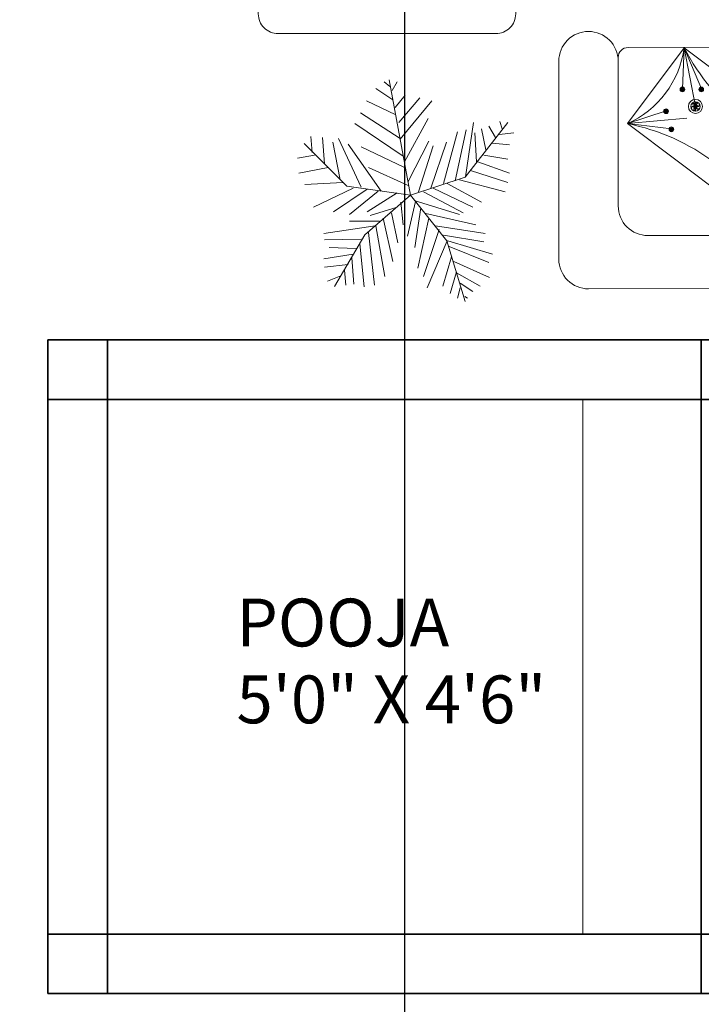
# Model space of a CAD drawing. Units: inches. Extents: x -61 to 1599, y -1316 to 257.
# Tile 22 of 204: x 365 to 434, y -1011 to -912. Entities that reach past the tile are written whole.
import ezdxf

# ---------------------------------------------------------------- set-up
doc = ezdxf.new("R2010")
doc.units = ezdxf.units.IN
doc.header["$MEASUREMENT"] = 0
for name, color, linetype, lineweight in [('A-ANNO-DIMS', 2, 'Continuous', 18), ('A-AREA-IDEN', 1, 'Continuous', 18), ('A-FLOR-CASE', 8, 'Continuous', 18), ('FURNITURE', 83, 'Continuous', 18), ('WALLS', 4, 'Continuous', 35)]:
    doc.layers.add(name, color=color, linetype=linetype, lineweight=lineweight)
doc.layers.add('FUR', color=83, linetype='Continuous')
doc.styles.get("Standard").update_dxf_attribs({"font": 'arial.ttf'})
doc.dimstyles.get("Standard").update_dxf_attribs({"dimtxt": 0.18, "dimasz": 0.18, "dimexe": 0.18, "dimexo": 0.0625, "dimgap": 0.09, "dimtad": 0, "dimtih": 1, "dimtoh": 1, "dimdec": 0, "dimzin": 0, "dimdsep": 46, "dimlunit": 3, "dimtxsty": 'Standard', "dimcen": 0.09, "dimadec": 0, "dimazin": 0, "dimtfac": 1, "dimtdec": 0, "dimtofl": 0, "dimtmove": 0, "dimatfit": 3, "dimfxl": 1, "dimtolj": 1, "dimtzin": 0, "dimarcsym": 0})

# ---------------------------------------------------------------- blocks, each defined once
blk = doc.blocks.new('*U264')
for p, q in [((-10.186, 53.64), (-13.084, 55.962)), ((0, 0), (-10.5, 57)), ((-9.099, 51.782), (-6.563, 55.962)), ((-8.737, 47.138), (-17.069, 52.711)), ((-7.65, 43.423), (-2.578, 49.46)), ((-7.288, 39.707), (-21.778, 46.673)), ((-5.839, 35.992), (4.667, 48.067)), ((-5.114, 27.632), (10.463, 46.673)), ((-5.114, 28.097), (-24.676, 40.636)), ((-3.665, 19.273), (-27.574, 35.527)), ((-2.941, 16.486), (8.652, 37.85)), ((27, 9), (48, 36)), ((27.127, 9.056), (31.112, 35.992)), ((38.719, 34.134), (41.979, 28.561)), ((44.153, 36.456), (45.239, 32.741)), ((16.259, 5.805), (23.142, 31.348)), ((22.055, 7.198), (27.489, 32.277)), ((31.836, 30.883), (32.561, 16.486)), ((35.096, 32.741), (37.27, 22.524)), ((43.791, 29.954), (51.036, 30.883)), ((-31.5, 4.5), (-52.5, 25.5)), ((-48.585, 21.131), (-49.309, 29.026)), ((-43.513, 28.561), (-42.427, 15.558)), ((-38.442, 26.239), (-34.819, 7.663)), ((-35.544, 28.097), (-24.314, 3.947)), ((-14.533, 2.09), (-30.834, 25.31)), ((-1.129, 6.734), (9.014, 26.704)), ((3.942, 1.625), (11.187, 24.381)), ((10.101, 3.483), (17.708, 26.239)), ((40.53, 25.775), (48.862, 24.846)), ((-47.498, 19.737), (-55.83, 18.344)), ((-24.314, 23.917), (-2.941, 13.7)), ((36.183, 19.737), (48.137, 17.88)), ((33.285, 16.486), (48.862, 10.913)), ((-40.615, 13.7), (-55.105, 10.913)), ((-20.691, 13.7), (-1.129, 4.876)), ((29.662, 12.307), (48.137, 6.269)), ((-33.37, 6.269), (-52.207, 5.34)), ((0, 0), (27, 9)), ((18.07, 5.805), (35.096, -3.483)), ((24.229, 7.663), (46.688, 1.625)), ((-28.299, 3.483), (-47.86, -5.805)), ((-21.416, 3.018), (-38.079, -8.128)), ((0, 0), (-31.5, 4.5)), ((-15.982, 2.09), (-30.11, -9.521)), ((0, 0), (-22.5, -19.5)), ((-6.563, 1.161), (-21.416, -8.128)), ((0, 0), (18, -22.5)), ((6.478, 1.625), (26.04, -8.592)), ((11.187, 3.483), (30.749, -5.805)), ((-4.752, -3.483), (-3.665, -14.629)), ((2.493, -3.019), (-1.491, -20.202)), ((1.769, -2.555), (24.229, -9.521)), ((-6.563, -5.805), (-19.967, -9.985)), ((-9.461, -8.592), (-6.201, -23.453)), ((5.029, -6.27), (2.131, -25.775)), ((7.565, -9.056), (32.198, -14.629)), ((-15.257, -12.772), (-30.11, -12.772)), ((-13.446, -11.378), (-8.737, -32.741)), ((9.014, -11.378), (3.58, -35.992)), ((-17.431, -15.094), (-42.789, -18.809)), ((-20.691, -18.345), (-17.793, -44.352)), ((-17.069, -15.094), (-12.721, -40.172)), ((14.085, -16.951), (6.478, -40.172)), ((12.274, -15.094), (36.907, -18.809)), ((-24.314, -21.596), (-42.427, -22.06)), ((-22.5, -19.5), (-37.5, -45)), ((-25.038, -23.918), (-22.865, -45.281)), ((18.07, -22.524), (8.289, -45.745)), ((16.259, -19.738), (36.183, -22.989)), ((18, -22.5), (27, -52.5)), ((18.433, -22.524), (40.53, -29.026)), ((-28.299, -29.026), (-42.789, -31.348)), ((-26.849, -26.24), (-40.253, -25.775)), ((19.157, -25.311), (38.719, -33.206)), ((-29.023, -30.884), (-27.936, -43.887)), ((20.244, -30.419), (15.897, -44.816)), ((21.331, -32.741), (39.081, -40.636)), ((-30.834, -34.135), (-42.427, -35.528)), ((-32.646, -36.921), (-31.921, -44.352)), ((22.78, -37.85), (19.519, -48.532)), ((22.78, -38.314), (34.372, -44.816)), ((-34.457, -39.708), (-40.978, -42.494)), ((24.591, -43.423), (30.749, -47.603)), ((24.591, -45.745), (23.142, -50.854)), ((26.764, -49.925), (28.213, -50.854))]:
    blk.add_line(p, q)
blk = doc.blocks.new('*U160')
at = {"layer": 'FUR'}
blk.add_open_spline([(0.005, 0.08), (-0.03, 0.048), (-0.098, -0.015), (0.075, -0.018), (0.024, -0.063), (0.005, -0.08)], degree=3, knots=[0, 0, 0, 0, 0.0954578, 0.1898773, 0.2470677, 0.2470677, 0.2470677, 0.2470677], dxfattribs=at)
blk = doc.blocks.new('*U161')
at = {"layer": 'FUR', "transparency": 16777216}
for p, rotation in [((222.173, -79.977), 60), ((222.178, -80.056), 120), ((222.25, -80.092), 180), ((222.312, -79.968), 300), ((222.317, -80.048), 240)]:
    blk.add_blockref('*U160', p, dxfattribs=dict(at, rotation=rotation))
blk.add_blockref('*U160', (222.24, -79.932), dxfattribs=at)
blk = doc.blocks.new('*U172')
at = {"layer": 'FUR'}
blk.add_open_spline([(0.005, 0.08), (-0.03, 0.048), (-0.098, -0.015), (0.075, -0.018), (0.024, -0.063), (0.005, -0.08)], degree=3, knots=[0, 0, 0, 0, 0.0954578, 0.1898773, 0.2470677, 0.2470677, 0.2470677, 0.2470677], dxfattribs=at)
blk = doc.blocks.new('*U173')
at = {"layer": 'FUR', "transparency": 16777216}
for p, rotation in [((222.173, -79.977), 60), ((222.178, -80.056), 120), ((222.25, -80.092), 180), ((222.312, -79.968), 300), ((222.317, -80.048), 240)]:
    blk.add_blockref('*U172', p, dxfattribs=dict(at, rotation=rotation))
blk.add_blockref('*U172', (222.24, -79.932), dxfattribs=at)
blk = doc.blocks.new('*U186')
at = {"layer": 'FUR'}
blk.add_open_spline([(0.005, 0.08), (-0.03, 0.048), (-0.098, -0.015), (0.075, -0.018), (0.024, -0.063), (0.005, -0.08)], degree=3, knots=[0, 0, 0, 0, 0.0954578, 0.1898773, 0.2470677, 0.2470677, 0.2470677, 0.2470677], dxfattribs=at)
blk = doc.blocks.new('*U187')
at = {"layer": 'FUR', "transparency": 16777216}
for p, rotation in [((222.173, -79.977), 60), ((222.178, -80.056), 120), ((222.25, -80.092), 180), ((222.312, -79.968), 300), ((222.317, -80.048), 240)]:
    blk.add_blockref('*U186', p, dxfattribs=dict(at, rotation=rotation))
blk.add_blockref('*U186', (222.24, -79.932), dxfattribs=at)
blk = doc.blocks.new('*U198')
at = {"layer": 'FUR'}
blk.add_open_spline([(0.005, 0.08), (-0.03, 0.048), (-0.098, -0.015), (0.075, -0.018), (0.024, -0.063), (0.005, -0.08)], degree=3, knots=[0, 0, 0, 0, 0.0954578, 0.1898773, 0.2470677, 0.2470677, 0.2470677, 0.2470677], dxfattribs=at)
blk = doc.blocks.new('*U199')
at = {"layer": 'FUR', "transparency": 16777216}
for p, rotation in [((222.173, -79.977), 60), ((222.178, -80.056), 120), ((222.25, -80.092), 180), ((222.312, -79.968), 300), ((222.317, -80.048), 240)]:
    blk.add_blockref('*U198', p, dxfattribs=dict(at, rotation=rotation))
blk.add_blockref('*U198', (222.24, -79.932), dxfattribs=at)
blk = doc.blocks.new('*U184')
at = {"layer": 'FUR'}
blk.add_open_spline([(0.015, 0.238), (-0.088, 0.143), (-0.292, -0.045), (0.224, -0.053), (0.072, -0.187), (0.015, -0.238)], degree=3, knots=[0, 0, 0, 0, 0.2846533, 0.5662105, 0.736751, 0.736751, 0.736751, 0.736751], dxfattribs=at)
blk = doc.blocks.new('*U159')
at = {"layer": 'FUR', "transparency": 16777216}
for p, rotation in [((662.517, -238.489), 60), ((662.531, -238.727), 120), ((662.745, -238.833), 180), ((662.929, -238.463), 300), ((662.944, -238.702), 240)]:
    blk.add_blockref('*U184', p, dxfattribs=dict(at, rotation=rotation))
blk.add_blockref('*U184', (662.716, -238.357), dxfattribs=at)
blk = doc.blocks.new('*U210')
at = {"layer": 'FUR'}
blk.add_open_spline([(0.015, 0.238), (-0.088, 0.143), (-0.292, -0.045), (0.224, -0.053), (0.072, -0.187), (0.015, -0.238)], degree=3, knots=[0, 0, 0, 0, 0.2846533, 0.5662105, 0.736751, 0.736751, 0.736751, 0.736751], dxfattribs=at)
blk = doc.blocks.new('*U185')
at = {"layer": 'FUR', "transparency": 16777216}
for p, rotation in [((662.517, -238.489), 60), ((662.531, -238.727), 120), ((662.745, -238.833), 180), ((662.929, -238.463), 300), ((662.944, -238.702), 240)]:
    blk.add_blockref('*U210', p, dxfattribs=dict(at, rotation=rotation))
blk.add_blockref('*U210', (662.716, -238.357), dxfattribs=at)
blk = doc.blocks.new('*U174')
at = {"layer": 'FUR'}
blk.add_open_spline([(0.005, 0.08), (-0.03, 0.048), (-0.098, -0.015), (0.075, -0.018), (0.024, -0.063), (0.005, -0.08)], degree=3, knots=[0, 0, 0, 0, 0.0954578, 0.1898773, 0.2470677, 0.2470677, 0.2470677, 0.2470677], dxfattribs=at)
blk = doc.blocks.new('*U175')
at = {"layer": 'FUR', "transparency": 16777216}
for p, rotation in [((222.173, -79.977), 60), ((222.178, -80.056), 120), ((222.25, -80.092), 180), ((222.312, -79.968), 300), ((222.317, -80.048), 240)]:
    blk.add_blockref('*U174', p, dxfattribs=dict(at, rotation=rotation))
blk.add_blockref('*U174', (222.24, -79.932), dxfattribs=at)
blk = doc.blocks.new('*U200')
at = {"layer": 'FUR'}
blk.add_open_spline([(0.005, 0.08), (-0.03, 0.048), (-0.098, -0.015), (0.075, -0.018), (0.024, -0.063), (0.005, -0.08)], degree=3, knots=[0, 0, 0, 0, 0.0954578, 0.1898773, 0.2470677, 0.2470677, 0.2470677, 0.2470677], dxfattribs=at)
blk = doc.blocks.new('*U201')
at = {"layer": 'FUR', "transparency": 16777216}
for p, rotation in [((222.173, -79.977), 60), ((222.178, -80.056), 120), ((222.25, -80.092), 180), ((222.312, -79.968), 300), ((222.317, -80.048), 240)]:
    blk.add_blockref('*U200', p, dxfattribs=dict(at, rotation=rotation))
blk.add_blockref('*U200', (222.24, -79.932), dxfattribs=at)
blk = doc.blocks.new('*U168')
at = {"layer": 'FUR'}
blk.add_open_spline([(0.015, 0.238), (-0.088, 0.143), (-0.292, -0.045), (0.224, -0.053), (0.072, -0.187), (0.015, -0.238)], degree=3, knots=[0, 0, 0, 0, 0.2846533, 0.5662105, 0.736751, 0.736751, 0.736751, 0.736751], dxfattribs=at)
blk = doc.blocks.new('*U169')
at = {"layer": 'FUR', "transparency": 16777216}
for p, rotation in [((662.517, -238.489), 60), ((662.531, -238.727), 120), ((662.745, -238.833), 180), ((662.929, -238.463), 300), ((662.944, -238.702), 240)]:
    blk.add_blockref('*U168', p, dxfattribs=dict(at, rotation=rotation))
blk.add_blockref('*U168', (662.716, -238.357), dxfattribs=at)
blk = doc.blocks.new('*U194')
at = {"layer": 'FUR'}
blk.add_open_spline([(0.015, 0.238), (-0.088, 0.143), (-0.292, -0.045), (0.224, -0.053), (0.072, -0.187), (0.015, -0.238)], degree=3, knots=[0, 0, 0, 0, 0.2846533, 0.5662105, 0.736751, 0.736751, 0.736751, 0.736751], dxfattribs=at)
blk = doc.blocks.new('*U195')
at = {"layer": 'FUR', "transparency": 16777216}
for p, rotation in [((662.517, -238.489), 60), ((662.531, -238.727), 120), ((662.745, -238.833), 180), ((662.929, -238.463), 300), ((662.944, -238.702), 240)]:
    blk.add_blockref('*U194', p, dxfattribs=dict(at, rotation=rotation))
blk.add_blockref('*U194', (662.716, -238.357), dxfattribs=at)
blk = doc.blocks.new('*U176')
at = {"layer": 'FUR'}
blk.add_open_spline([(0.005, 0.08), (-0.03, 0.048), (-0.098, -0.015), (0.075, -0.018), (0.024, -0.063), (0.005, -0.08)], degree=3, knots=[0, 0, 0, 0, 0.0954578, 0.1898773, 0.2470677, 0.2470677, 0.2470677, 0.2470677], dxfattribs=at)
blk = doc.blocks.new('*U177')
at = {"layer": 'FUR', "transparency": 16777216}
for p, rotation in [((222.173, -79.977), 60), ((222.178, -80.056), 120), ((222.25, -80.092), 180), ((222.312, -79.968), 300), ((222.317, -80.048), 240)]:
    blk.add_blockref('*U176', p, dxfattribs=dict(at, rotation=rotation))
blk.add_blockref('*U176', (222.24, -79.932), dxfattribs=at)
blk = doc.blocks.new('*U202')
at = {"layer": 'FUR'}
blk.add_open_spline([(0.005, 0.08), (-0.03, 0.048), (-0.098, -0.015), (0.075, -0.018), (0.024, -0.063), (0.005, -0.08)], degree=3, knots=[0, 0, 0, 0, 0.0954578, 0.1898773, 0.2470677, 0.2470677, 0.2470677, 0.2470677], dxfattribs=at)
blk = doc.blocks.new('*U203')
at = {"layer": 'FUR', "transparency": 16777216}
for p, rotation in [((222.173, -79.977), 60), ((222.178, -80.056), 120), ((222.25, -80.092), 180), ((222.312, -79.968), 300), ((222.317, -80.048), 240)]:
    blk.add_blockref('*U202', p, dxfattribs=dict(at, rotation=rotation))
blk.add_blockref('*U202', (222.24, -79.932), dxfattribs=at)
blk = doc.blocks.new('*U170')
at = {"layer": 'FUR'}
blk.add_open_spline([(0.015, 0.238), (-0.088, 0.143), (-0.292, -0.045), (0.224, -0.053), (0.072, -0.187), (0.015, -0.238)], degree=3, knots=[0, 0, 0, 0, 0.2846533, 0.5662105, 0.736751, 0.736751, 0.736751, 0.736751], dxfattribs=at)
blk = doc.blocks.new('*U171')
at = {"layer": 'FUR', "transparency": 16777216}
for p, rotation in [((662.517, -238.489), 60), ((662.531, -238.727), 120), ((662.745, -238.833), 180), ((662.929, -238.463), 300), ((662.944, -238.702), 240)]:
    blk.add_blockref('*U170', p, dxfattribs=dict(at, rotation=rotation))
blk.add_blockref('*U170', (662.716, -238.357), dxfattribs=at)
blk = doc.blocks.new('*U196')
at = {"layer": 'FUR'}
blk.add_open_spline([(0.015, 0.238), (-0.088, 0.143), (-0.292, -0.045), (0.224, -0.053), (0.072, -0.187), (0.015, -0.238)], degree=3, knots=[0, 0, 0, 0, 0.2846533, 0.5662105, 0.736751, 0.736751, 0.736751, 0.736751], dxfattribs=at)
blk = doc.blocks.new('*U197')
at = {"layer": 'FUR', "transparency": 16777216}
for p, rotation in [((662.517, -238.489), 60), ((662.531, -238.727), 120), ((662.745, -238.833), 180), ((662.929, -238.463), 300), ((662.944, -238.702), 240)]:
    blk.add_blockref('*U196', p, dxfattribs=dict(at, rotation=rotation))
blk.add_blockref('*U196', (662.716, -238.357), dxfattribs=at)
blk = doc.blocks.new('*U164')
at = {"layer": 'FUR'}
blk.add_open_spline([(0.005, 0.08), (-0.03, 0.048), (-0.098, -0.015), (0.075, -0.018), (0.024, -0.063), (0.005, -0.08)], degree=3, knots=[0, 0, 0, 0, 0.0954578, 0.1898773, 0.2470677, 0.2470677, 0.2470677, 0.2470677], dxfattribs=at)
blk = doc.blocks.new('*U165')
at = {"layer": 'FUR', "transparency": 16777216}
for p, rotation in [((222.173, -79.977), 60), ((222.178, -80.056), 120), ((222.25, -80.092), 180), ((222.312, -79.968), 300), ((222.317, -80.048), 240)]:
    blk.add_blockref('*U164', p, dxfattribs=dict(at, rotation=rotation))
blk.add_blockref('*U164', (222.24, -79.932), dxfattribs=at)
blk = doc.blocks.new('*U190')
at = {"layer": 'FUR'}
blk.add_open_spline([(0.005, 0.08), (-0.03, 0.048), (-0.098, -0.015), (0.075, -0.018), (0.024, -0.063), (0.005, -0.08)], degree=3, knots=[0, 0, 0, 0, 0.0954578, 0.1898773, 0.2470677, 0.2470677, 0.2470677, 0.2470677], dxfattribs=at)
blk = doc.blocks.new('*U191')
at = {"layer": 'FUR', "transparency": 16777216}
for p, rotation in [((222.173, -79.977), 60), ((222.178, -80.056), 120), ((222.25, -80.092), 180), ((222.312, -79.968), 300), ((222.317, -80.048), 240)]:
    blk.add_blockref('*U190', p, dxfattribs=dict(at, rotation=rotation))
blk.add_blockref('*U190', (222.24, -79.932), dxfattribs=at)
blk = doc.blocks.new('*U183')
at = {"layer": 'FUR'}
blk.add_open_spline([(0.015, 0.238), (-0.088, 0.143), (-0.292, -0.045), (0.224, -0.053), (0.072, -0.187), (0.015, -0.238)], degree=3, knots=[0, 0, 0, 0, 0.2846533, 0.5662105, 0.736751, 0.736751, 0.736751, 0.736751], dxfattribs=at)
blk = doc.blocks.new('*U162')
at = {"layer": 'FUR', "transparency": 16777216}
for p, rotation in [((662.517, -238.489), 60), ((662.531, -238.727), 120), ((662.745, -238.833), 180), ((662.929, -238.463), 300), ((662.944, -238.702), 240)]:
    blk.add_blockref('*U183', p, dxfattribs=dict(at, rotation=rotation))
blk.add_blockref('*U183', (662.716, -238.357), dxfattribs=at)
blk = doc.blocks.new('*U209')
at = {"layer": 'FUR'}
blk.add_open_spline([(0.015, 0.238), (-0.088, 0.143), (-0.292, -0.045), (0.224, -0.053), (0.072, -0.187), (0.015, -0.238)], degree=3, knots=[0, 0, 0, 0, 0.2846533, 0.5662105, 0.736751, 0.736751, 0.736751, 0.736751], dxfattribs=at)
blk = doc.blocks.new('*U188')
at = {"layer": 'FUR', "transparency": 16777216}
for p, rotation in [((662.517, -238.489), 60), ((662.531, -238.727), 120), ((662.745, -238.833), 180), ((662.929, -238.463), 300), ((662.944, -238.702), 240)]:
    blk.add_blockref('*U209', p, dxfattribs=dict(at, rotation=rotation))
blk.add_blockref('*U209', (662.716, -238.357), dxfattribs=at)
blk = doc.blocks.new('*U182')
at = {"layer": 'FUR'}
blk.add_open_spline([(0.005, 0.08), (-0.03, 0.048), (-0.098, -0.015), (0.075, -0.018), (0.024, -0.063), (0.005, -0.08)], degree=3, knots=[0, 0, 0, 0, 0.0954578, 0.1898773, 0.2470677, 0.2470677, 0.2470677, 0.2470677], dxfattribs=at)
blk = doc.blocks.new('*U163')
at = {"layer": 'FUR', "transparency": 16777216}
for p, rotation in [((222.173, -79.977), 60), ((222.178, -80.056), 120), ((222.25, -80.092), 180), ((222.312, -79.968), 300), ((222.317, -80.048), 240)]:
    blk.add_blockref('*U182', p, dxfattribs=dict(at, rotation=rotation))
blk.add_blockref('*U182', (222.24, -79.932), dxfattribs=at)
blk = doc.blocks.new('*U208')
at = {"layer": 'FUR'}
blk.add_open_spline([(0.005, 0.08), (-0.03, 0.048), (-0.098, -0.015), (0.075, -0.018), (0.024, -0.063), (0.005, -0.08)], degree=3, knots=[0, 0, 0, 0, 0.0954578, 0.1898773, 0.2470677, 0.2470677, 0.2470677, 0.2470677], dxfattribs=at)
blk = doc.blocks.new('*U189')
at = {"layer": 'FUR', "transparency": 16777216}
for p, rotation in [((222.173, -79.977), 60), ((222.178, -80.056), 120), ((222.25, -80.092), 180), ((222.312, -79.968), 300), ((222.317, -80.048), 240)]:
    blk.add_blockref('*U208', p, dxfattribs=dict(at, rotation=rotation))
blk.add_blockref('*U208', (222.24, -79.932), dxfattribs=at)
blk = doc.blocks.new('*U166')
at = {"layer": 'FUR'}
blk.add_open_spline([(0.015, 0.238), (-0.088, 0.143), (-0.292, -0.045), (0.224, -0.053), (0.072, -0.187), (0.015, -0.238)], degree=3, knots=[0, 0, 0, 0, 0.2846533, 0.5662105, 0.736751, 0.736751, 0.736751, 0.736751], dxfattribs=at)
blk = doc.blocks.new('*U167')
at = {"layer": 'FUR', "transparency": 16777216}
for p, rotation in [((662.517, -238.489), 60), ((662.531, -238.727), 120), ((662.745, -238.833), 180), ((662.929, -238.463), 300), ((662.944, -238.702), 240)]:
    blk.add_blockref('*U166', p, dxfattribs=dict(at, rotation=rotation))
blk.add_blockref('*U166', (662.716, -238.357), dxfattribs=at)
blk = doc.blocks.new('*U192')
at = {"layer": 'FUR'}
blk.add_open_spline([(0.015, 0.238), (-0.088, 0.143), (-0.292, -0.045), (0.224, -0.053), (0.072, -0.187), (0.015, -0.238)], degree=3, knots=[0, 0, 0, 0, 0.2846533, 0.5662105, 0.736751, 0.736751, 0.736751, 0.736751], dxfattribs=at)
blk = doc.blocks.new('*U193')
at = {"layer": 'FUR', "transparency": 16777216}
for p, rotation in [((662.517, -238.489), 60), ((662.531, -238.727), 120), ((662.745, -238.833), 180), ((662.929, -238.463), 300), ((662.944, -238.702), 240)]:
    blk.add_blockref('*U192', p, dxfattribs=dict(at, rotation=rotation))
blk.add_blockref('*U192', (662.716, -238.357), dxfattribs=at)
blk = doc.blocks.new('*U178')
at = {"layer": 'FUR'}
blk.add_open_spline([(0.005, 0.08), (-0.03, 0.048), (-0.098, -0.015), (0.075, -0.018), (0.024, -0.063), (0.005, -0.08)], degree=3, knots=[0, 0, 0, 0, 0.0954578, 0.1898773, 0.2470677, 0.2470677, 0.2470677, 0.2470677], dxfattribs=at)
blk = doc.blocks.new('*U179')
at = {"layer": 'FUR', "transparency": 16777216}
for p, rotation in [((222.173, -79.977), 60), ((222.178, -80.056), 120), ((222.25, -80.092), 180), ((222.312, -79.968), 300), ((222.317, -80.048), 240)]:
    blk.add_blockref('*U178', p, dxfattribs=dict(at, rotation=rotation))
blk.add_blockref('*U178', (222.24, -79.932), dxfattribs=at)
blk = doc.blocks.new('*U180')
at = {"layer": 'FUR'}
blk.add_open_spline([(0.005, 0.08), (-0.03, 0.048), (-0.098, -0.015), (0.075, -0.018), (0.024, -0.063), (0.005, -0.08)], degree=3, knots=[0, 0, 0, 0, 0.0954578, 0.1898773, 0.2470677, 0.2470677, 0.2470677, 0.2470677], dxfattribs=at)
blk = doc.blocks.new('*U181')
at = {"layer": 'FUR', "transparency": 16777216}
for p, rotation in [((222.173, -79.977), 60), ((222.178, -80.056), 120), ((222.25, -80.092), 180), ((222.312, -79.968), 300), ((222.317, -80.048), 240)]:
    blk.add_blockref('*U180', p, dxfattribs=dict(at, rotation=rotation))
blk.add_blockref('*U180', (222.24, -79.932), dxfattribs=at)
blk = doc.blocks.new('*U204')
at = {"layer": 'FUR'}
blk.add_open_spline([(0.005, 0.08), (-0.03, 0.048), (-0.098, -0.015), (0.075, -0.018), (0.024, -0.063), (0.005, -0.08)], degree=3, knots=[0, 0, 0, 0, 0.0954578, 0.1898773, 0.2470677, 0.2470677, 0.2470677, 0.2470677], dxfattribs=at)
blk = doc.blocks.new('*U205')
at = {"layer": 'FUR', "transparency": 16777216}
for p, rotation in [((222.173, -79.977), 60), ((222.178, -80.056), 120), ((222.25, -80.092), 180), ((222.312, -79.968), 300), ((222.317, -80.048), 240)]:
    blk.add_blockref('*U204', p, dxfattribs=dict(at, rotation=rotation))
blk.add_blockref('*U204', (222.24, -79.932), dxfattribs=at)
blk = doc.blocks.new('*U206')
at = {"layer": 'FUR'}
blk.add_open_spline([(0.005, 0.08), (-0.03, 0.048), (-0.098, -0.015), (0.075, -0.018), (0.024, -0.063), (0.005, -0.08)], degree=3, knots=[0, 0, 0, 0, 0.0954578, 0.1898773, 0.2470677, 0.2470677, 0.2470677, 0.2470677], dxfattribs=at)
blk = doc.blocks.new('*U207')
at = {"layer": 'FUR', "transparency": 16777216}
for p, rotation in [((222.173, -79.977), 60), ((222.178, -80.056), 120), ((222.25, -80.092), 180), ((222.312, -79.968), 300), ((222.317, -80.048), 240)]:
    blk.add_blockref('*U206', p, dxfattribs=dict(at, rotation=rotation))
blk.add_blockref('*U206', (222.24, -79.932), dxfattribs=at)
blk = doc.blocks.new('SOFA-LOVESEAT')
for p, q in [((22.442, 54), (5.47, 54)), ((14.776, 53.751), (14.253, 49.285)), ((14.776, 53.751), (15.332, 47.757)), ((14.776, 53.751), (16.081, 49.817)), ((22.442, 54), (26, 54)), ((3.47, 8), (3.47, 52)), ((24.442, 52), (24.442, 32)), ((16.029, 49.837), (15.869, 49.837)), ((16.029, 49.837), (16.189, 49.837)), ((14.201, 49.305), (14.041, 49.305)), ((14.201, 49.305), (14.36, 49.305)), ((15.332, 47.757), (14.855, 47.757)), ((15.332, 47.757), (15.808, 47.757)), ((22.422, 48.013), (16.511, 46.872)), ((18.228, 48.187), (18.068, 48.187)), ((18.228, 48.187), (18.388, 48.187)), ((22.422, 48.013), (18.28, 48.167)), ((22.422, 48.013), (18.28, 46.263)), ((16.511, 46.872), (16.035, 46.872)), ((16.511, 46.872), (16.988, 46.872)), ((18.228, 46.282), (18.068, 46.282)), ((18.228, 46.282), (18.388, 46.282)), ((12.946, 43.35), (12.47, 43.35)), ((12.946, 43.35), (13.423, 43.35)), ((3.47, 38.686), (7.612, 40.436)), ((3.47, 38.686), (9.381, 39.828)), ((7.56, 40.455), (7.4, 40.455)), ((7.56, 40.455), (7.719, 40.455)), ((9.381, 39.828), (8.904, 39.828)), ((9.381, 39.828), (9.857, 39.828)), ((10.561, 38.942), (10.084, 38.942)), ((11.116, 32.948), (10.561, 38.942)), ((10.561, 38.942), (11.037, 38.942)), ((3.47, 38.686), (7.612, 38.532)), ((7.56, 38.551), (7.4, 38.551)), ((7.56, 38.551), (7.719, 38.551)), ((9.759, 36.901), (9.599, 36.901)), ((9.759, 36.901), (9.918, 36.901)), ((11.116, 32.948), (9.811, 36.882)), ((11.116, 32.948), (11.639, 37.414)), ((11.587, 37.433), (11.427, 37.433)), ((11.587, 37.433), (11.747, 37.433)), ((22.442, 30), (3.47, 30)), ((22.442, 30), (22.442, 30)), ((24.442, 8), (24.442, 28)), ((11.116, 27.026), (9.811, 23.092)), ((11.116, 27.026), (10.561, 21.032)), ((11.116, 27.026), (11.639, 22.56)), ((9.759, 23.073), (9.599, 23.073)), ((9.759, 23.073), (9.918, 23.073)), ((11.587, 22.541), (11.427, 22.541)), ((11.587, 22.541), (11.747, 22.541)), ((3.47, 21.288), (7.612, 21.442)), ((3.47, 21.288), (9.381, 20.146)), ((3.47, 21.288), (7.612, 19.538)), ((7.56, 21.423), (7.4, 21.423)), ((7.56, 21.423), (7.719, 21.423)), ((10.561, 21.032), (10.084, 21.032)), ((10.561, 21.032), (11.037, 21.032)), ((9.381, 20.146), (8.904, 20.146)), ((9.381, 20.146), (9.857, 20.146)), ((7.56, 19.518), (7.4, 19.518)), ((7.56, 19.518), (7.719, 19.518)), ((12.946, 16.624), (12.47, 16.624)), ((12.946, 16.624), (13.423, 16.624)), ((16.511, 13.102), (16.035, 13.102)), ((22.422, 11.961), (16.511, 13.102)), ((16.511, 13.102), (16.988, 13.102)), ((18.228, 13.691), (18.068, 13.691)), ((18.228, 13.691), (18.388, 13.691)), ((22.422, 11.961), (18.28, 13.711)), ((14.776, 6.223), (15.332, 12.217)), ((15.332, 12.217), (14.855, 12.217)), ((15.332, 12.217), (15.808, 12.217)), ((22.422, 11.961), (18.28, 11.807)), ((18.228, 11.787), (18.068, 11.787)), ((18.228, 11.787), (18.388, 11.787)), ((14.201, 10.669), (14.041, 10.669)), ((14.201, 10.669), (14.36, 10.669)), ((14.776, 6.223), (14.253, 10.689)), ((14.776, 6.223), (16.081, 10.156)), ((16.029, 10.137), (15.869, 10.137)), ((16.029, 10.137), (16.189, 10.137)), ((22.442, 6), (5.47, 6)), ((22.442, 6), (26, 6))]:
    blk.add_line(p, q)
blk.add_lwpolyline([(26, 6), (26, 2, -0.414214), (24, 0), (2, 0, -0.414214), (0, 2), (0, 58, -0.414213), (2, 60), (24, 60, -0.414214), (26, 58), (26, 54)], format="xyb")
for points in [[(11.116, 32.948), (22.422, 48.013), (14.776, 53.751), (3.47, 38.686)], [(11.116, 27.026), (22.422, 11.961), (14.776, 6.223), (3.47, 21.288)]]:
    blk.add_lwpolyline(points, close=True)
for centre, radius in [((16.029, 49.837), 0.238), ((16.029, 49.837), 0.16), ((14.201, 49.305), 0.238), ((14.201, 49.305), 0.16), ((15.332, 47.757), 0.71), ((15.332, 47.757), 0.476), ((18.228, 48.187), 0.238), ((18.228, 48.187), 0.16), ((16.511, 46.872), 0.71), ((16.511, 46.872), 0.476), ((18.228, 46.282), 0.238), ((18.228, 46.282), 0.16), ((12.946, 43.35), 0.71), ((12.946, 43.35), 0.476), ((7.56, 40.455), 0.238), ((7.56, 40.455), 0.16), ((9.381, 39.828), 0.71), ((9.381, 39.828), 0.476), ((7.56, 38.551), 0.238), ((10.561, 38.942), 0.71), ((10.561, 38.942), 0.476), ((7.56, 38.551), 0.16), ((9.759, 36.901), 0.238), ((9.759, 36.901), 0.16), ((11.587, 37.433), 0.238), ((11.587, 37.433), 0.16), ((9.759, 23.073), 0.238), ((9.759, 23.073), 0.16), ((11.587, 22.541), 0.238), ((11.587, 22.541), 0.16), ((7.56, 21.423), 0.238), ((7.56, 21.423), 0.16), ((10.561, 21.032), 0.71), ((10.561, 21.032), 0.476), ((9.381, 20.146), 0.71), ((9.381, 20.146), 0.476), ((7.56, 19.518), 0.238), ((7.56, 19.518), 0.16), ((12.946, 16.624), 0.71), ((12.946, 16.624), 0.476), ((18.228, 13.691), 0.238), ((16.511, 13.102), 0.71), ((16.511, 13.102), 0.476), ((18.228, 13.691), 0.16), ((15.332, 12.217), 0.71), ((15.332, 12.217), 0.476), ((18.228, 11.787), 0.238), ((18.228, 11.787), 0.16), ((14.201, 10.669), 0.238), ((14.201, 10.669), 0.16), ((16.029, 10.137), 0.238), ((16.029, 10.137), 0.16)]:
    blk.add_circle(centre, radius)
for centre, radius, start, end in [((5.47, 52), 2, 90, 180.00002), ((-6.541, 57.974), 21.731, 297.43166, 348.79559), ((23.745, 57.74), 9.816, 203.97425, 262.253), ((22.442, 52), 2, 0, 90), ((32.433, 28.726), 21.731, 117.43166, 168.79559), ((2.147, 28.96), 9.816, 23.97425, 82.253), ((22.442, 32), 2, 270, 0), ((22.442, 28), 2, 0, 90), ((2.147, 31.014), 9.816, 277.74703, 336.02578), ((32.433, 31.248), 21.731, 191.20444, 242.56837), ((-6.541, 2), 21.731, 11.20444, 62.56837), ((23.745, 2.234), 9.816, 97.74703, 156.02578), ((5.47, 8), 2, 180.00002, 270), ((22.442, 8), 2, 270, 0)]:
    blk.add_arc(centre, radius, start, end)
at = {"xscale": -1, "rotation": 90.00003000000098}
for name, p in [('*U189', (-63.984, 272.082)), ('*U191', (-65.812, 271.55)), ('*U188', (-223.264, 710.487)), ('*U205', (-61.785, 270.431)), ('*U193', (-222.084, 709.602)), ('*U207', (-61.785, 268.527)), ('*U197', (-225.649, 706.08)), ('*U187', (-72.453, 262.7)), ('*U185', (-229.215, 702.558)), ('*U195', (-228.035, 701.672)), ('*U199', (-72.453, 260.796)), ('*U201', (-70.254, 259.146)), ('*U203', (-68.426, 259.678))]:
    blk.add_blockref(name, p, dxfattribs=at)
at = {"rotation": 90}
for name, p in [('*U175', (-70.254, -199.172)), ('*U177', (-68.425, -199.704)), ('*U173', (-72.453, -200.822)), ('*U169', (-228.034, -641.698)), ('*U159', (-229.214, -642.584)), ('*U161', (-72.453, -202.727)), ('*U171', (-225.649, -646.106)), ('*U167', (-222.084, -649.628)), ('*U181', (-61.785, -208.554)), ('*U162', (-223.264, -650.513)), ('*U179', (-61.785, -210.458)), ('*U165', (-65.812, -211.576)), ('*U163', (-63.983, -212.108))]:
    blk.add_blockref(name, p, dxfattribs=at)
blk = doc.blocks.new('*U514')
at = {"layer": 'FUR'}
blk.add_open_spline([(0.005, 0.08), (-0.03, 0.048), (-0.098, -0.015), (0.075, -0.018), (0.024, -0.063), (0.005, -0.08)], degree=3, knots=[0, 0, 0, 0, 0.0954578, 0.1898773, 0.2470677, 0.2470677, 0.2470677, 0.2470677], dxfattribs=at)
blk = doc.blocks.new('*U515')
at = {"layer": 'FUR', "transparency": 16777216}
for p, rotation in [((222.173, -79.977), 60), ((222.178, -80.056), 120), ((222.25, -80.092), 180), ((222.312, -79.968), 300), ((222.317, -80.048), 240)]:
    blk.add_blockref('*U514', p, dxfattribs=dict(at, rotation=rotation))
blk.add_blockref('*U514', (222.24, -79.932), dxfattribs=at)
blk = doc.blocks.new('*U516')
at = {"layer": 'FUR'}
blk.add_open_spline([(0.005, 0.08), (-0.03, 0.048), (-0.098, -0.015), (0.075, -0.018), (0.024, -0.063), (0.005, -0.08)], degree=3, knots=[0, 0, 0, 0, 0.0954578, 0.1898773, 0.2470677, 0.2470677, 0.2470677, 0.2470677], dxfattribs=at)
blk = doc.blocks.new('*U517')
at = {"layer": 'FUR', "transparency": 16777216}
for p, rotation in [((222.173, -79.977), 60), ((222.178, -80.056), 120), ((222.25, -80.092), 180), ((222.312, -79.968), 300), ((222.317, -80.048), 240)]:
    blk.add_blockref('*U516', p, dxfattribs=dict(at, rotation=rotation))
blk.add_blockref('*U516', (222.24, -79.932), dxfattribs=at)
blk = doc.blocks.new('*U510')
at = {"layer": 'FUR'}
blk.add_open_spline([(0.005, 0.08), (-0.03, 0.048), (-0.098, -0.015), (0.075, -0.018), (0.024, -0.063), (0.005, -0.08)], degree=3, knots=[0, 0, 0, 0, 0.0954578, 0.1898773, 0.2470677, 0.2470677, 0.2470677, 0.2470677], dxfattribs=at)
blk = doc.blocks.new('*U511')
at = {"layer": 'FUR', "transparency": 16777216}
for p, rotation in [((222.173, -79.977), 60), ((222.178, -80.056), 120), ((222.25, -80.092), 180), ((222.312, -79.968), 300), ((222.317, -80.048), 240)]:
    blk.add_blockref('*U510', p, dxfattribs=dict(at, rotation=rotation))
blk.add_blockref('*U510', (222.24, -79.932), dxfattribs=at)
blk = doc.blocks.new('*U479')
at = {"layer": 'FUR'}
blk.add_open_spline([(0.015, 0.238), (-0.088, 0.143), (-0.292, -0.045), (0.224, -0.053), (0.072, -0.187), (0.015, -0.238)], degree=3, knots=[0, 0, 0, 0, 0.2846533, 0.5662105, 0.736751, 0.736751, 0.736751, 0.736751], dxfattribs=at)
blk = doc.blocks.new('*U480')
at = {"layer": 'FUR', "transparency": 16777216}
for p, rotation in [((662.517, -238.489), 60), ((662.531, -238.727), 120), ((662.745, -238.833), 180), ((662.929, -238.463), 300), ((662.944, -238.702), 240)]:
    blk.add_blockref('*U479', p, dxfattribs=dict(at, rotation=rotation))
blk.add_blockref('*U479', (662.716, -238.357), dxfattribs=at)
blk = doc.blocks.new('*U512')
at = {"layer": 'FUR'}
blk.add_open_spline([(0.005, 0.08), (-0.03, 0.048), (-0.098, -0.015), (0.075, -0.018), (0.024, -0.063), (0.005, -0.08)], degree=3, knots=[0, 0, 0, 0, 0.0954578, 0.1898773, 0.2470677, 0.2470677, 0.2470677, 0.2470677], dxfattribs=at)
blk = doc.blocks.new('*U513')
at = {"layer": 'FUR', "transparency": 16777216}
for p, rotation in [((222.173, -79.977), 60), ((222.178, -80.056), 120), ((222.25, -80.092), 180), ((222.312, -79.968), 300), ((222.317, -80.048), 240)]:
    blk.add_blockref('*U512', p, dxfattribs=dict(at, rotation=rotation))
blk.add_blockref('*U512', (222.24, -79.932), dxfattribs=at)
blk = doc.blocks.new('SOFA-THREE-SEAT-ALT-2')
for p, q in [((30, 24.442), (6.996, 24.38)), ((12.664, 24.333), (12.509, 20.191)), ((12.664, 24.333), (13.805, 18.423)), ((12.664, 24.333), (14.414, 20.191)), ((6, 23), (5.999, 23.377)), ((12.49, 20.139), (12.49, 20.299)), ((12.49, 20.139), (12.49, 19.979)), ((14.394, 20.139), (14.394, 20.299)), ((14.394, 20.139), (14.394, 19.979)), ((13.805, 18.423), (13.805, 18.899)), ((6.926, 16.687), (10.859, 17.993)), ((10.84, 17.94), (10.84, 18.1)), ((10.84, 17.94), (10.84, 17.78)), ((13.805, 18.423), (13.805, 17.946)), ((6.926, 16.687), (12.92, 17.243)), ((6.926, 16.687), (11.391, 16.164)), ((11.372, 16.112), (11.372, 16.272)), ((11.372, 16.112), (11.372, 15.952))]:
    blk.add_line(p, q)
blk.add_lwpolyline([(78, 8.382), (78, 23, -0.414214), (81, 26), (81, 26, -0.414214), (84, 23), (84, 3, -0.414214), (81, 0), (3, 0, -0.414214), (0, 3), (0, 23, -0.414214), (3, 26), (3, 26, -0.414214), (6, 23), (6, 8.382, 0.414214), (9, 5.382), (75, 5.382, 0.414214)], format="xyb", close=True)
blk.add_lwpolyline([(27.729, 13.028), (12.664, 24.333), (6.926, 16.687), (21.991, 5.382)], close=True)
for centre, radius in [((12.49, 20.139), 0.238), ((12.49, 20.139), 0.16), ((14.394, 20.139), 0.238), ((14.394, 20.139), 0.16), ((13.805, 18.423), 0.71), ((13.805, 18.423), 0.476), ((10.84, 17.94), 0.238), ((10.84, 17.94), 0.16), ((11.372, 16.112), 0.238), ((11.372, 16.112), 0.16)]:
    blk.add_circle(centre, radius)
for centre, radius, start, end in [((6.999, 23.38), 1, 90.15417, 180.15417), ((2.937, 25.656), 9.816, 293.97422, 352.25297), ((31.951, 34.344), 21.731, 207.43163, 258.79556), ((2.703, -4.63), 21.731, 27.43163, 78.79556)]:
    blk.add_arc(centre, radius, start, end)
at = {"xscale": -1, "rotation": 180}
for name, p in [('*U511', (-209.755, -59.873)), ('*U513', (-207.851, -59.873)), ('*U480', (-648.925, -220.173)), ('*U515', (-211.405, -62.072)), ('*U517', (-210.873, -63.901))]:
    blk.add_blockref(name, p, dxfattribs=at)
blk = doc.blocks.new('*D696')
at = {"layer": 'A-ANNO-DIMS', "color": 0, "lineweight": -2, "transparency": 16777216}
for p, q in [((690.64, -873.169), (-61.077, -873.169)), ((-60.897, -873.349), (-60.897, -1025.799)), ((-60.897, -1178.613), (-60.897, -1026.163)), ((690.64, -1178.793), (-61.077, -1178.793))]:
    blk.add_line(p, q, dxfattribs=at)
at = {"layer": 'A-ANNO-DIMS', "color": 0, "transparency": 16777216}
for points in [[(-60.927, -873.349), (-60.867, -873.349), (-60.897, -873.169)], [(-60.927, -1178.613), (-60.867, -1178.613), (-60.897, -1178.793)]]:
    blk.add_solid(points, dxfattribs=at)
at = {"layer": 'DEFPOINTS', "color": 0, "transparency": 16777216}
for p in [(-60.897, -873.169), (690.703, -873.169), (690.703, -1178.793)]:
    blk.add_point(p, dxfattribs=at)
at = {"layer": 'A-ANNO-DIMS', "color": 0, "transparency": 16777216, "insert": (-60.897, -1025.981), "char_height": 0.18, "attachment_point": 5}
blk.add_mtext('\\A1;305.6', dxfattribs=at)
blk = doc.blocks.new('*D710')
at = {"layer": 'A-ANNO-DIMS', "color": 0, "lineweight": -2, "transparency": 16777216}
for p, q in [((319.703, -465.385), (319.703, -1315.725)), ((403.703, -465.385), (403.703, -1315.725)), ((319.883, -1315.545), (361.484, -1315.545)), ((403.523, -1315.545), (361.921, -1315.545))]:
    blk.add_line(p, q, dxfattribs=at)
at = {"layer": 'A-ANNO-DIMS', "color": 0, "transparency": 16777216}
for points in [[(319.883, -1315.515), (319.883, -1315.575), (319.703, -1315.545)], [(403.523, -1315.515), (403.523, -1315.575), (403.703, -1315.545)]]:
    blk.add_solid(points, dxfattribs=at)
at = {"layer": 'DEFPOINTS', "color": 0, "transparency": 16777216}
for p in [(319.703, -465.323), (403.703, -465.323), (403.703, -1315.545)]:
    blk.add_point(p, dxfattribs=at)
at = {"layer": 'A-ANNO-DIMS', "color": 0, "transparency": 16777216, "insert": (361.703, -1315.545), "char_height": 0.18, "attachment_point": 5}
blk.add_mtext('\\A1;84', dxfattribs=at)

msp = doc.modelspace()

# ---------------------------------------------------------------- linework, layer by layer
at = {"layer": 'A-FLOR-CASE'}
msp.add_lwpolyline([(433.7028, -1003.9446), (421.7505, -1003.9446), (421.7505, -949.9446), (433.7028, -949.9446)], close=True, dxfattribs=at)
at = {"layer": 'WALLS'}
for p, q in [((367.7028, -943.9446), (403.7028, -943.9446)), ((367.7028, -1009.9446), (367.7028, -943.9446)), ((373.7028, -1009.9446), (373.7028, -943.9446)), ((397.7028, -943.9446), (544.7028, -943.9446)), ((433.7028, -1009.9446), (433.7028, -943.9446)), ((367.7028, -949.9446), (373.7028, -949.9446)), ((373.7028, -949.9446), (433.7028, -949.9446)), ((433.7028, -949.9446), (439.7028, -949.9446)), ((367.7028, -1003.9446), (544.7028, -1003.9446)), ((367.7028, -1009.9446), (544.7028, -1009.9446))]:
    msp.add_line(p, q, dxfattribs=at)

# ---------------------------------------------------------------- block references
at = {"layer": 'FURNITURE'}
msp.add_blockref('SOFA-LOVESEAT', (388.9518, -913.0047), dxfattribs=at)
at = {"layer": 'FURNITURE', "rotation": 0.0183708733775309}
msp.add_blockref('SOFA-THREE-SEAT-ALT-2', (419.3112, -938.7885), dxfattribs=at)
at = {"layer": 'FURNITURE', "xscale": 0.2045054661246738, "yscale": 0.2045054661246738, "zscale": 0.2045054661246738}
msp.add_blockref('*U264', (404.3297, -929.3337), dxfattribs=at)

# ---------------------------------------------------------------- texts
at = {"layer": 'A-AREA-IDEN'}
for s, height, p in [('POOJA', 4.8321, (386.7531, -974.9022)), ('5\'0" X 4\'6"', 4.832098, (386.7531, -982.6646))]:
    msp.add_text(s, height=height, dxfattribs=at).set_placement(p)

# ---------------------------------------------------------------- dimensions: what is measured, and where the dimension line sits
at = {"layer": 'A-ANNO-DIMS'}
dim = msp.add_linear_dim(base=(403.7028, -1315.5446), p1=(319.7028, -465.3229), p2=(403.7028, -465.3229), dimstyle='Standard', override={"dimdec": 0, "dimlfac": 1, "dimrnd": 0, "dimzin": 0, "dimdsep": 46, "dimlunit": 2}, dxfattribs=at)
dim.commit()
dim.dimension.update_dxf_attribs({"geometry": '*D710', "text_midpoint": (361.7028, -1315.5446)})
dim = msp.add_linear_dim(base=(-60.8972, -873.169), p1=(690.7028, -1178.7933), p2=(690.7028, -873.169), angle=90, dimstyle='Standard', override={"dimdec": 1, "dimlfac": 1, "dimrnd": 0, "dimzin": 0, "dimdsep": 46, "dimlunit": 2}, dxfattribs=at)
dim.commit()
dim.dimension.update_dxf_attribs({"geometry": '*D696', "text_midpoint": (-60.8972, -1025.9812)})

doc.saveas('drawing.dxf')
